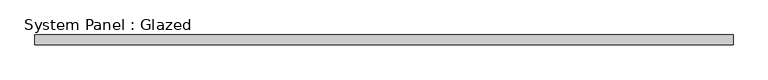
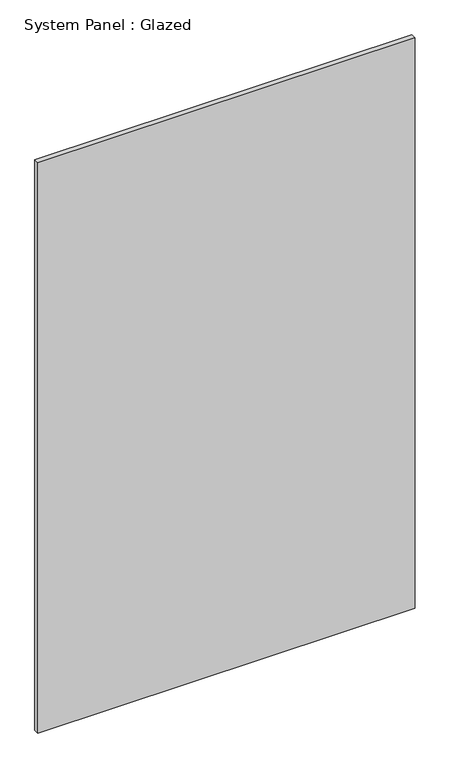
"""IFC4 building model written with IfcOpenShell, lengths in millimetres: plate geometry, System Panel : Glazed."""

from ifc_helpers import new_model, si_unit, origin, origin_with_axes, place, context, project, spatial, polyline, outline, extrude, source, transform, mapped, element, save


def system_panel_glazed_97c7e3fb(model_context):
    return source(origin(), model_context, "Body", "SweptSolid", [
        extrude(outline(polyline([(914.4, 19.05), (-914.4, 19.05), (-914.4, 44.45), (914.4, 44.45), (914.4, 19.05)])), origin_with_axes(), (0.0, 0.0, 1.0), 2921.0),
    ])


if __name__ == "__main__":
    model = new_model("IFC4")
    model_context = context("Model", 3, world=origin())
    ifc_project = project(units=[si_unit("LENGTHUNIT", "METRE", prefix="MILLI")], contexts=[model_context])
    site = spatial("IfcSite", under=ifc_project)
    building = spatial("IfcBuilding", under=site)
    placement = place(None, origin())
    system_panel_glazed_shape = system_panel_glazed_97c7e3fb(model_context)
    element("IfcPlate", 1, ObjectType="System Panel : Glazed", at=placement, inside=building, context=model_context, shape_type="MappedRepresentation", body=[
        mapped(system_panel_glazed_shape, transform((0.0, 0.0, 0.0), x_axis=(1.0, 0.0, 0.0), y_axis=(0.0, 1.0, 0.0), z_axis=(0.0, 0.0, 1.0))),
    ])
    save(model, "model.ifc")

# Revit data of these elements
# Type "System Panel : Glazed"
#   Construction Type Id = "GSP4R"
#   Analytic Construction = "1/8 in Pilkington single glazing"
#   Visual Light Transmittance = 0.9
#   Solar Heat Gain Coefficient = 0.86
#   Heat Transfer Coefficient (U) = 1.18115 BTU/(h·ft²·°F)
# Element 1 (IfcPlate, "System Panel : Glazed")
#   Materials on its faces: "Glass"
# Materials
#   "Glass": class "Glass", colour RGB 0 128 192, transparency 0.75, Description = "Soda Lime Glass", Cost = 0
